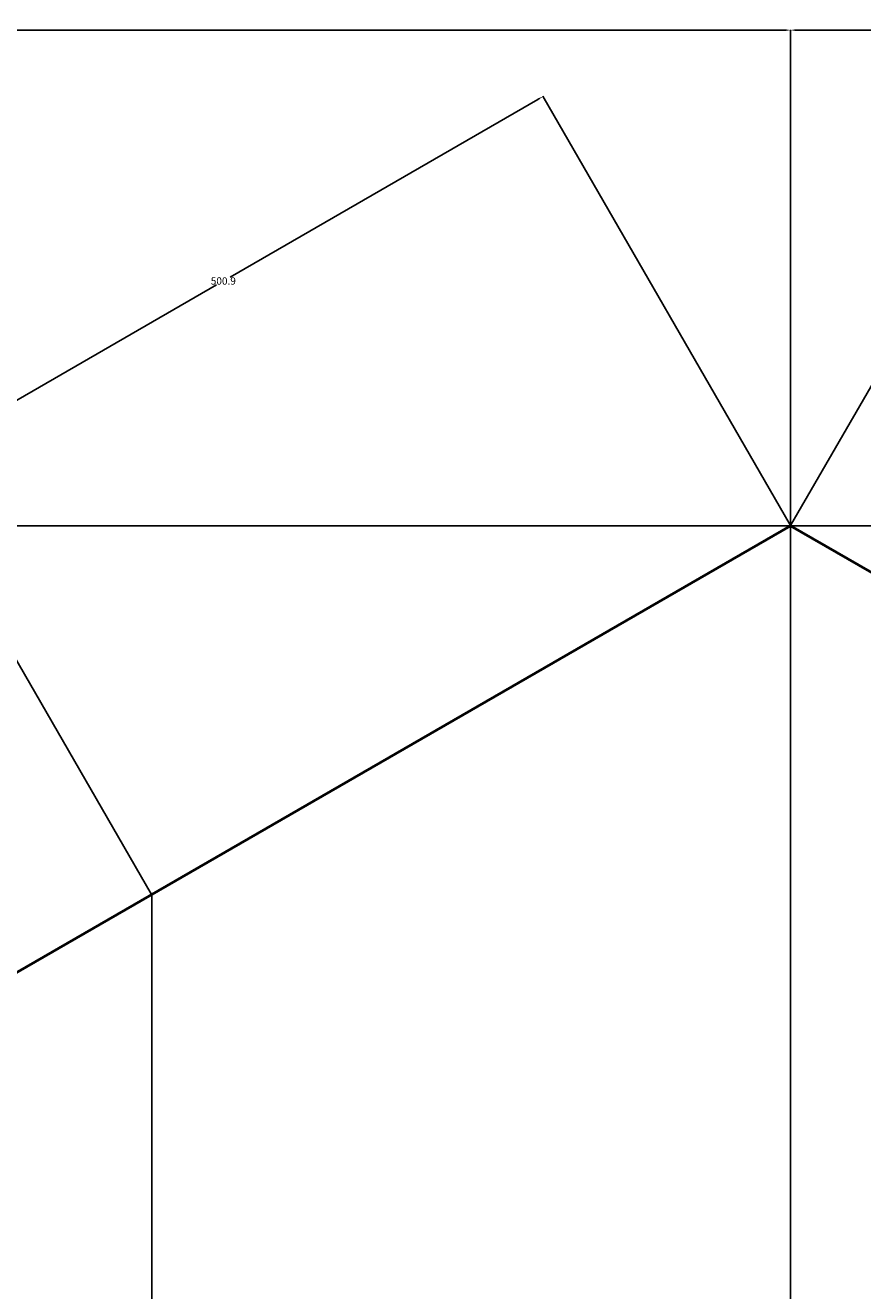
# Model space of a CAD drawing. Units: metres. Extents: x -2391 to 4922, y -635 to 4845.
# Tile 27 of 37: x 31 to 600, y 3986 to 4845. Entities that reach past the tile are written whole.
import ezdxf

# ---------------------------------------------------------------- set-up
doc = ezdxf.new("R2010")
doc.units = ezdxf.units.M
doc.header["$MEASUREMENT"] = 0
for name, color, linetype, lineweight in [('A-ANNO-DIMS', 2, 'Continuous', 18), ('A-FLOR-FIXT', 3, 'Continuous', 25), ('A-WALL', 7, 'Continuous', 50)]:
    doc.layers.add(name, color=color, linetype=linetype, lineweight=lineweight)
doc.styles.get("Standard").update_dxf_attribs({"font": 'arial.ttf'})
doc.dimstyles.get("Standard").update_dxf_attribs({"dimtxt": 5, "dimasz": 4, "dimexe": 0.18, "dimexo": 0.0625, "dimgap": 0.09, "dimtad": 0, "dimtih": 1, "dimtoh": 1, "dimdec": 0, "dimzin": 0, "dimdsep": 46, "dimtxsty": 'Standard', "dimcen": 0.09, "dimadec": 0, "dimazin": 0, "dimtfac": 1, "dimtdec": 0, "dimtofl": 0, "dimtmove": 0, "dimatfit": 3, "dimfxl": 1, "dimtolj": 1, "dimtzin": 0, "dimarcsym": 0})

# ---------------------------------------------------------------- blocks, each defined once
blk = doc.blocks.new('*D9')
at = {"layer": 'A-ANNO-DIMS', "color": 0, "lineweight": -2, "transparency": 16777216}
for p, q in [((-2047.33, 3005.34), (-2047.33, 4841.96)), ((-2043.33, 4841.78), (-755.9, 4841.78)), ((546.74, 4841.78), (-740.69, 4841.78)), ((550.74, 4505.34), (550.74, 4841.96))]:
    blk.add_line(p, q, dxfattribs=at)
at = {"layer": 'A-ANNO-DIMS', "color": 0, "transparency": 16777216}
for points in [[(-2043.33, 4842.44), (-2043.33, 4841.11), (-2047.33, 4841.78)], [(546.74, 4842.44), (546.74, 4841.11), (550.74, 4841.78)]]:
    blk.add_solid(points, dxfattribs=at)
at = {"layer": 'Defpoints', "color": 0, "transparency": 16777216}
for p in [(550.74, 4841.78), (550.74, 4505.28), (-2047.33, 3005.28)]:
    blk.add_point(p, dxfattribs=at)
at = {"layer": 'A-ANNO-DIMS', "color": 0, "transparency": 16777216, "insert": (-748.3, 4841.78), "char_height": 5, "attachment_point": 5}
blk.add_mtext('\\A1;2598', dxfattribs=at)
blk = doc.blocks.new('*D10')
at = {"layer": 'A-ANNO-DIMS', "color": 0, "lineweight": -2, "transparency": 16777216}
for p, q in [((550.68, 4505.28), (-2384.01, 4505.28)), ((-2383.83, 4501.28), (-2383.83, 2107.92)), ((-2383.83, -290.72), (-2383.83, 2102.63)), ((-488.55, -294.72), (-2384.01, -294.72))]:
    blk.add_line(p, q, dxfattribs=at)
at = {"layer": 'A-ANNO-DIMS', "color": 0, "transparency": 16777216}
for points in [[(-2384.5, 4501.28), (-2383.17, 4501.28), (-2383.83, 4505.28)], [(-2384.5, -290.72), (-2383.17, -290.72), (-2383.83, -294.72)]]:
    blk.add_solid(points, dxfattribs=at)
at = {"layer": 'Defpoints', "color": 0, "transparency": 16777216}
for p in [(-2383.83, 4505.28), (550.74, 4505.28), (-488.49, -294.72)]:
    blk.add_point(p, dxfattribs=at)
at = {"layer": 'A-ANNO-DIMS', "color": 0, "transparency": 16777216, "insert": (-2383.83, 2105.28), "char_height": 5, "attachment_point": 5}
blk.add_mtext('\\A1;4800', dxfattribs=at)
blk = doc.blocks.new('*D11')
at = {"layer": 'A-ANNO-DIMS', "color": 0, "lineweight": -2, "transparency": 16777216}
for p, q in [((550.8, 4505.28), (887.42, 4505.28)), ((887.24, 4501.28), (887.24, 3317.92)), ((887.24, 2129.28), (887.24, 3312.63)), ((550.8, 2125.28), (887.42, 2125.28))]:
    blk.add_line(p, q, dxfattribs=at)
at = {"layer": 'A-ANNO-DIMS', "color": 0, "transparency": 16777216}
for points in [[(886.58, 4501.28), (887.91, 4501.28), (887.24, 4505.28)], [(886.58, 2129.28), (887.91, 2129.28), (887.24, 2125.28)]]:
    blk.add_solid(points, dxfattribs=at)
at = {"layer": 'Defpoints', "color": 0, "transparency": 16777216}
for p in [(550.74, 4505.28), (550.74, 2125.28), (887.24, 2125.28)]:
    blk.add_point(p, dxfattribs=at)
at = {"layer": 'A-ANNO-DIMS', "color": 0, "transparency": 16777216, "insert": (887.24, 3315.28), "char_height": 5, "attachment_point": 5}
blk.add_mtext('\\A1;2380', dxfattribs=at)
blk = doc.blocks.new('*D17')
at = {"layer": 'A-ANNO-DIMS', "color": 0, "lineweight": -2, "transparency": 16777216}
for p, q in [((550.74, 3005.34), (550.74, 4841.96)), ((554.74, 4841.78), (1014.86, 4841.78)), ((1492.03, 4841.78), (1031.91, 4841.78)), ((1496.03, 2662.52), (1496.03, 4841.96))]:
    blk.add_line(p, q, dxfattribs=at)
at = {"layer": 'A-ANNO-DIMS', "color": 0, "transparency": 16777216}
for points in [[(554.74, 4842.44), (554.74, 4841.11), (550.74, 4841.78)], [(1492.03, 4842.44), (1492.03, 4841.11), (1496.03, 4841.78)]]:
    blk.add_solid(points, dxfattribs=at)
at = {"layer": 'Defpoints', "color": 0, "transparency": 16777216}
for p in [(1496.03, 4841.78), (550.74, 3005.28), (1496.03, 2662.46)]:
    blk.add_point(p, dxfattribs=at)
at = {"layer": 'A-ANNO-DIMS', "color": 0, "transparency": 16777216, "insert": (1023.39, 4841.78), "char_height": 5, "attachment_point": 5}
blk.add_mtext('\\A1;945.3', dxfattribs=at)
blk = doc.blocks.new('*D34')
at = {"layer": 'A-ANNO-DIMS', "color": 0, "lineweight": -2, "transparency": 16777216}
for p, q in [((550.77, 4505.33), (719.08, 4796.85)), ((722.46, 4794.69), (745.06, 4781.65)), ((776.81, 4763.31), (754.21, 4776.36)), ((612.05, 4469.95), (780.36, 4761.47))]:
    blk.add_line(p, q, dxfattribs=at)
at = {"layer": 'A-ANNO-DIMS', "color": 0, "transparency": 16777216}
for points in [[(722.79, 4795.27), (722.12, 4794.12), (718.99, 4796.69)], [(777.14, 4763.89), (776.48, 4762.74), (780.27, 4761.31)]]:
    blk.add_solid(points, dxfattribs=at)
at = {"layer": 'Defpoints', "color": 0, "transparency": 16777216}
for p in [(780.27, 4761.31), (550.74, 4505.28), (612.02, 4469.9)]:
    blk.add_point(p, dxfattribs=at)
at = {"layer": 'A-ANNO-DIMS', "color": 0, "transparency": 16777216, "insert": (749.63, 4779), "char_height": 5, "attachment_point": 5}
blk.add_mtext('\\A1;70.76', dxfattribs=at)
blk = doc.blocks.new('*D39')
at = {"layer": 'A-ANNO-DIMS', "color": 0, "lineweight": -2, "transparency": 16777216}
for p, q in [((116.89, 4254.86), (-51.42, 4546.38)), ((-54.79, 4544.23), (-241.56, 4436.4)), ((-437.49, 4323.28), (-250.72, 4431.11)), ((-272.74, 4029.91), (-441.05, 4321.43))]:
    blk.add_line(p, q, dxfattribs=at)
at = {"layer": 'A-ANNO-DIMS', "color": 0, "transparency": 16777216}
for points in [[(-55.13, 4544.81), (-54.46, 4543.65), (-51.33, 4546.23)], [(-437.82, 4323.85), (-437.16, 4322.7), (-440.96, 4321.28)]]:
    blk.add_solid(points, dxfattribs=at)
at = {"layer": 'Defpoints', "color": 0, "transparency": 16777216}
for p in [(-51.33, 4546.23), (116.92, 4254.81), (-272.71, 4029.86)]:
    blk.add_point(p, dxfattribs=at)
at = {"layer": 'A-ANNO-DIMS', "color": 0, "transparency": 16777216, "insert": (-246.14, 4433.75), "char_height": 5, "attachment_point": 5}
blk.add_mtext('\\A1;449.9', dxfattribs=at)
blk = doc.blocks.new('*D40')
at = {"layer": 'A-ANNO-DIMS', "color": 0, "lineweight": -2, "transparency": 16777216}
for p, q in [((379.03, 4794.69), (170.16, 4674.1)), ((550.71, 4505.33), (382.4, 4796.85)), ((-47.86, 4548.23), (161, 4668.82)), ((116.89, 4254.86), (-51.42, 4546.38))]:
    blk.add_line(p, q, dxfattribs=at)
at = {"layer": 'A-ANNO-DIMS', "color": 0, "transparency": 16777216}
for points in [[(378.69, 4795.27), (379.36, 4794.12), (382.49, 4796.69)], [(-48.2, 4548.81), (-47.53, 4547.65), (-51.33, 4546.23)]]:
    blk.add_solid(points, dxfattribs=at)
at = {"layer": 'Defpoints', "color": 0, "transparency": 16777216}
for p in [(382.49, 4796.69), (550.74, 4505.28), (116.92, 4254.81)]:
    blk.add_point(p, dxfattribs=at)
at = {"layer": 'A-ANNO-DIMS', "color": 0, "transparency": 16777216, "insert": (165.58, 4671.46), "char_height": 5, "attachment_point": 5}
blk.add_mtext('\\A1;500.9', dxfattribs=at)

msp = doc.modelspace()

# ---------------------------------------------------------------- linework, layer by layer
at = {"layer": 'A-FLOR-FIXT'}
msp.add_line((116.9223, 3504.8104), (116.9223, 4254.8104), dxfattribs=at)
at = {"layer": 'A-WALL'}
for p, q in [((-1008.1038, 3605.2763), (550.7419, 4505.2763)), ((550.7419, 4505.2763), (3607.8116, 2740.2763))]:
    msp.add_line(p, q, dxfattribs=at)

# ---------------------------------------------------------------- dimensions: what is measured, and where the dimension line sits
at = {"layer": 'A-ANNO-DIMS'}
for base, p1, p2, override, picture, middle in [((550.7419, 4841.7763), (-2047.3343, 3005.2763), (550.7419, 4505.2763), {"dimdec": 0, "dimlfac": 1, "dimrnd": 0, "dimzin": 0, "dimdsep": 46, "dimlunit": 2}, '*D9', (-748.2962, 4841.7763)), ((1496.0309, 4841.7763), (550.7419, 3005.2763), (1496.0309, 2662.4566), {"dimdec": 1, "dimlfac": 1, "dimrnd": 0, "dimzin": 0, "dimdsep": 46, "dimlunit": 2}, '*D17', (1023.3864, 4841.7763))]:
    dim = msp.add_linear_dim(base=base, p1=p1, p2=p2, dimstyle='Standard', override=override, dxfattribs=at)
    dim.commit()
    dim.dimension.update_dxf_attribs({"geometry": picture, "text_midpoint": middle})
for base, p1, p2, angle, override, picture, middle in [((382.4919, 4796.6938), (116.9223, 4254.8104), (550.7419, 4505.2763), 30, {"dimdec": 1, "dimlfac": 1, "dimrnd": 0, "dimzin": 0, "dimdsep": 46, "dimlunit": 2}, '*D40', (165.5821, 4671.4609)), ((780.2733, 4761.313), (550.7419, 4505.2763), (612.0233, 4469.8954), 330, {"dimdec": 2, "dimlfac": 1, "dimrnd": 0, "dimzin": 0, "dimdsep": 46, "dimlunit": 2}, '*D34', (749.6326, 4779.0034)), ((-51.3277, 4546.228), (-272.7053, 4029.8588), (116.9223, 4254.8104), 30, {"dimdec": 1, "dimlfac": 1, "dimrnd": 0, "dimzin": 0, "dimdsep": 46, "dimlunit": 2}, '*D39', (-246.1415, 4433.7522)), ((-2383.8343, 4505.2763), (-488.4886, -294.7237), (550.7419, 4505.2763), 90, {"dimdec": 0, "dimlfac": 1, "dimrnd": 0, "dimzin": 0, "dimdsep": 46, "dimlunit": 2}, '*D10', (-2383.8343, 2105.2763)), ((887.2419, 2125.2763), (550.7419, 4505.2763), (550.7419, 2125.2763), 270, {"dimdec": 0, "dimlfac": 1, "dimrnd": 0, "dimzin": 0, "dimdsep": 46, "dimlunit": 2}, '*D11', (887.2419, 3315.2763))]:
    dim = msp.add_linear_dim(base=base, p1=p1, p2=p2, angle=angle, dimstyle='Standard', override=override, dxfattribs=at)
    dim.commit()
    dim.dimension.update_dxf_attribs({"geometry": picture, "text_midpoint": middle})

doc.saveas('drawing.dxf')
